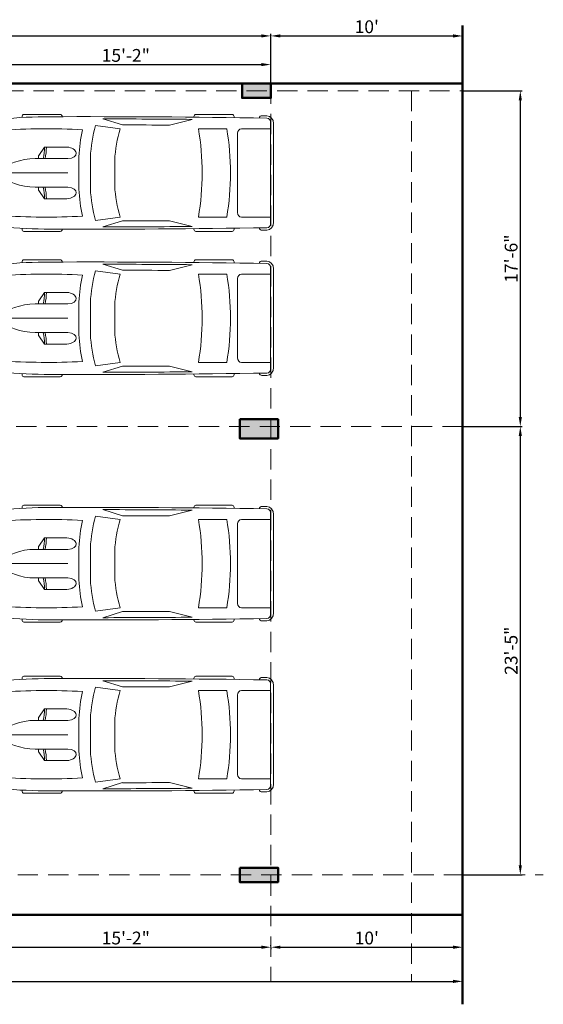
# Model space of a CAD drawing. Units: millimetres. Extents: x 1706 to 5913, y 156 to 1716.
# Tile 7 of 26: x 2350 to 2678, y 1086 to 1702. Entities that reach past the tile are written whole.
import ezdxf

# ---------------------------------------------------------------- set-up
doc = ezdxf.new("R2010")
doc.units = ezdxf.units.MM
doc.linetypes.add('DASHED', pattern=[19.05, 12.7, -6.35])
for name, color, linetype, lineweight in [('A-ANNO-DIMS', 2, 'Continuous', 18), ('A-COLS', 20, 'Continuous', 50), ('A-EQPM', 8, 'Continuous', 18), ('A-FLOR-OVHD', 9, 'DASHED', 18), ('A-WALL', 7, 'Continuous', 50)]:
    doc.layers.add(name, color=color, linetype=linetype, lineweight=lineweight)
doc.styles.get("Standard").update_dxf_attribs({"font": 'arial.ttf'})
doc.dimstyles.new('ISO-25', dxfattribs={"dimtxt": 8, "dimasz": 6, "dimexe": 1.25, "dimexo": 0.625, "dimtad": 1, "dimdec": 0, "dimlunit": 3, "dimtxsty": 'Standard', "dimcen": 2.5, "dimadec": 0, "dimazin": 0, "dimtfac": 1, "dimtdec": 0, "dimtmove": 0, "dimatfit": 3, "dimfxl": 1, "dimarcsym": 0})

# ---------------------------------------------------------------- blocks, each defined once
blk = doc.blocks.new('*U10')
for p, q in [((21.1, 37.41), (21.1, 36.83)), ((46.55, 38.89), (22.35, 38.89)), ((47.8, 37.39), (47.8, 37.41)), ((87.99, 31.87), (74.76, 35.92)), ((134.31, 35.6), (119.29, 31.78)), ((135.45, 37.07), (135.45, 37.41)), ((136.7, 38.89), (160.9, 38.89)), ((162.15, 37.41), (162.15, 36.77)), ((186.47, -33.5), (186.47, 33.5)), ((188.4, -32.76), (188.4, 32.76)), ((70.03, 31.54), (86.41, 29.35)), ((138.42, 29.35), (157.25, 29.35)), ((164.52, 26.39), (164.52, -26.39)), ((186.47, 29.35), (167.01, 29.35)), ((32.27, 11.63), (36.13, 17.17)), ((36.13, 17.17), (50.94, 17.17)), ((29.77, 9.51), (51.68, 9.51)), ((32.12, 9.51), (32.12, 11.15)), ((58.92, -10.77), (58.92, 10.77)), ((66.55, -10.53), (66.55, 10.53)), ((82.74, 8.5), (82.74, -8.5)), ((186.47, -10.53), (186.47, 10.53)), ((3.27, 6.13), (0.1, 0.41)), ((0, 0), (51.68, 0)), ((0.1, -0.41), (3.27, -6.13)), ((29.77, -9.51), (51.68, -9.51)), ((32.12, -9.51), (32.12, -11.15)), ((32.27, -11.63), (36.13, -17.17)), ((36.13, -17.17), (50.94, -17.17)), ((86.41, -29.35), (70.03, -31.54)), ((87.99, -31.87), (74.76, -35.92)), ((134.31, -35.6), (119.29, -31.78)), ((157.25, -29.35), (138.42, -29.35)), ((167.01, -29.35), (186.47, -29.35)), ((21.1, -37.41), (21.1, -36.83)), ((46.55, -38.89), (22.35, -38.89)), ((47.8, -37.39), (47.8, -37.41)), ((135.45, -37.07), (135.45, -37.41)), ((136.7, -38.89), (160.9, -38.89)), ((162.15, -37.41), (162.15, -36.77))]:
    blk.add_line(p, q)
for centre, major_axis, ratio, start_param, end_param in [((266.03, -27.52), (0, 313.31), 0.842304, 1.367076, 1.39176), ((41.19, -490.86), (0, 528.23), 0.842304, 0.00281, 0.075598), ((22.35, 37.41), (0, -1.48), 0.842304, 3.141593, 4.712389), ((64.48, -10555.62), (0, 10593.03), 0.842304, -0.013397, 0.002797), ((46.55, 37.41), (0, 1.48), 0.842304, -1.570796, 0), ((64.48, -10555.62), (0, -10591.55), 0.842304, 3.133765, 3.140441), ((136.7, 37.41), (0, -1.48), 0.842304, 3.141593, 4.712389), ((160.9, 37.41), (0, 1.48), 0.842304, -1.570796, 0), ((180.63, 35.84), (0, 2.22), 0.842304, -0.013017, 1.249894), ((64.48, -10556.36), (0, 10595.31), 0.842304, -0.013397, -0.013017), ((183.98, 33.5), (0, -2.96), 0.842304, 1.570796, 3.128196), ((183.98, 32.76), (0, -5.25), 0.842304, 1.570796, 3.128196), ((259.18, -27.52), (0, -305.3), 0.842304, 4.528606, 4.561838), ((37.47, -593.96), (0, -623.33), 0.842304, 3.096046, 3.200911), ((134.4, 5.39), (0, -89.78), 0.842304, 4.449482, 4.652344), ((135.29, 5.39), (0, 81.77), 0.842304, 1.245306, 1.50788), ((149.6, 2.8), (0, -79.58), 0.842304, 4.372215, 4.640744), ((95.79, -3666.35), (0, -3698.24), 0.842304, 3.134049, 3.144098), ((17.08, 0), (0, 147.02), 0.842304, 4.511394, 4.913384), ((35.91, 0), (0, 147.02), 0.842304, 4.511394, 4.913384), ((167.01, 26.39), (0, 2.96), 0.842304, 0, 1.570796), ((-204.49, 52.4), (0, -250.96), 0.842304, 1.385369, 1.434372), ((13.04, 17.01), (0, 27.42), 0.842304, 4.435146, 4.718221), ((14.2, 17.01), (0, 27.42), 0.842304, 4.435146, 4.718221), ((50.79, 13.34), (6.34, -0.36), 0.603834, -1.395552, 1.581315), ((29.77, -46.66), (0, 56.17), 0.842304, 0, 0.590319), ((32.75, 11.15), (0, 0.74), 0.842304, 0.879714, 1.570796), ((0.62, 0), (0, -0.74), 0.842304, 4.131459, 5.293319), ((-204.49, -52.4), (0, 250.96), 0.842304, -1.434372, -1.385369), ((29.77, 46.66), (0, 56.17), 0.842304, 2.551274, 3.141593), ((32.75, -11.15), (0, -0.74), 0.842304, 4.712389, 5.403472), ((13.04, -17.01), (0, -27.42), 0.842304, 1.564964, 1.848039), ((14.2, -17.01), (0, -27.42), 0.842304, 1.564964, 1.848039), ((134.4, -5.39), (0, -89.78), 0.842304, -1.510751, -1.307889), ((135.29, -5.39), (0, -81.77), 0.842304, -1.50788, -1.245306), ((149.6, -2.8), (0, -79.58), 0.842304, -1.499151, -1.230623), ((259.18, 27.52), (0, 305.3), 0.842304, 1.721348, 1.754579), ((266.03, 27.52), (0, 313.31), 0.842304, 1.749832, 1.774517), ((37.47, 593.96), (0, -623.33), 0.842304, -0.059319, 0.045547), ((95.79, 3666.35), (0, -3698.24), 0.842304, -0.002505, 0.007544), ((167.01, -26.39), (0, -2.96), 0.842304, 4.712389, 6.283185), ((41.19, 490.86), (0, -528.23), 0.842304, -0.075598, -0.00281), ((22.35, -37.41), (0, 1.48), 0.842304, 1.570796, 3.141593), ((64.48, 10555.62), (0, 10593.03), 0.842304, 3.138796, 3.15499), ((46.55, -37.41), (0, -1.48), 0.842304, 0, 1.570796), ((64.48, 10555.62), (0, -10591.55), 0.842304, 0.001152, 0.007828), ((136.7, -37.41), (0, -1.48), 0.842304, -1.570796, 0), ((160.9, -37.41), (0, 1.48), 0.842304, 3.141593, 4.712389), ((180.63, -35.84), (0, -2.22), 0.842304, -1.249894, 0.013017), ((64.48, 10556.36), (0, 10595.31), 0.842304, 3.15461, 3.15499), ((183.98, -33.5), (0, 2.96), 0.842304, 3.15499, 4.712389), ((183.98, -32.76), (0, -5.25), 0.842304, 0.013397, 1.570796)]:
    blk.add_ellipse(centre, major_axis=major_axis, ratio=ratio, start_param=start_param, end_param=end_param)
at = {"extrusion": (0, 0, -1)}
blk.add_ellipse((50.79, -13.34), major_axis=(6.34, 0.36), ratio=0.603834, start_param=-1.395552, end_param=1.581315, dxfattribs=at)
blk = doc.blocks.new('*D90')
at = {"layer": 'A-ANNO-DIMS', "color": 0, "lineweight": -2, "transparency": 16777216}
for p, q in [((2325.9, 1122.72), (2325.9, 1123.34)), ((2331.9, 1122.09), (2501.4, 1122.09)), ((2507.4, 1122.72), (2507.4, 1123.34))]:
    blk.add_line(p, q, dxfattribs=at)
at = {"layer": 'A-ANNO-DIMS', "color": 0, "transparency": 16777216}
for points in [[(2331.9, 1123.09), (2331.9, 1121.09), (2325.9, 1122.09)], [(2501.4, 1123.09), (2501.4, 1121.09), (2507.4, 1122.09)]]:
    blk.add_solid(points, dxfattribs=at)
at = {"layer": 'Defpoints', "color": 0, "transparency": 16777216}
for p in [(2325.9, 1122.09), (2507.4, 1122.09), (2507.4, 1122.09)]:
    blk.add_point(p, dxfattribs=at)
at = {"layer": 'A-ANNO-DIMS', "color": 0, "transparency": 16777216, "insert": (2416.65, 1126.8), "char_height": 8, "attachment_point": 5}
blk.add_mtext('15\'-2"', dxfattribs=at)
blk = doc.blocks.new('*D91')
at = {"layer": 'A-ANNO-DIMS', "color": 0, "lineweight": -2, "transparency": 16777216}
for p, q in [((2507.4, 1121.47), (2507.4, 1120.84)), ((2513.4, 1122.09), (2621.4, 1122.09)), ((2627.4, 1123.72), (2627.4, 1120.84))]:
    blk.add_line(p, q, dxfattribs=at)
at = {"layer": 'A-ANNO-DIMS', "color": 0, "transparency": 16777216}
for points in [[(2513.4, 1123.09), (2513.4, 1121.09), (2507.4, 1122.09)], [(2621.4, 1123.09), (2621.4, 1121.09), (2627.4, 1122.09)]]:
    blk.add_solid(points, dxfattribs=at)
at = {"layer": 'Defpoints', "color": 0, "transparency": 16777216}
for p in [(2507.4, 1122.09), (2627.4, 1124.34), (2627.4, 1122.09)]:
    blk.add_point(p, dxfattribs=at)
at = {"layer": 'A-ANNO-DIMS', "color": 0, "transparency": 16777216, "insert": (2567.4, 1126.8), "char_height": 8, "attachment_point": 5}
blk.add_mtext("10'", dxfattribs=at)
blk = doc.blocks.new('*D96')
at = {"layer": 'A-ANNO-DIMS', "color": 0, "lineweight": -2, "transparency": 16777216}
for p, q in [((2325.9, 1662.9), (2325.9, 1675.38)), ((2507.4, 1662.9), (2507.4, 1675.38)), ((2331.9, 1674.13), (2501.4, 1674.13))]:
    blk.add_line(p, q, dxfattribs=at)
at = {"layer": 'A-ANNO-DIMS', "color": 0, "transparency": 16777216}
for points in [[(2331.9, 1675.13), (2331.9, 1673.13), (2325.9, 1674.13)], [(2501.4, 1675.13), (2501.4, 1673.13), (2507.4, 1674.13)]]:
    blk.add_solid(points, dxfattribs=at)
at = {"layer": 'Defpoints', "color": 0, "transparency": 16777216}
for p in [(2507.4, 1674.13), (2325.9, 1662.28), (2507.4, 1662.28)]:
    blk.add_point(p, dxfattribs=at)
at = {"layer": 'A-ANNO-DIMS', "color": 0, "transparency": 16777216, "insert": (2416.65, 1678.84), "char_height": 8, "attachment_point": 5}
blk.add_mtext('15\'-2"', dxfattribs=at)
blk = doc.blocks.new('*D83')
at = {"layer": 'A-ANNO-DIMS', "color": 0, "lineweight": -2, "transparency": 16777216}
for p, q in [((2507.4, 1692.67), (2507.4, 1693.3)), ((2513.4, 1692.05), (2621.4, 1692.05)), ((2627.4, 1692.67), (2627.4, 1693.3))]:
    blk.add_line(p, q, dxfattribs=at)
at = {"layer": 'A-ANNO-DIMS', "color": 0, "transparency": 16777216}
for points in [[(2513.4, 1693.05), (2513.4, 1691.05), (2507.4, 1692.05)], [(2621.4, 1693.05), (2621.4, 1691.05), (2627.4, 1692.05)]]:
    blk.add_solid(points, dxfattribs=at)
at = {"layer": 'Defpoints', "color": 0, "transparency": 16777216}
for p in [(2507.4, 1692.05), (2627.4, 1692.05), (2627.4, 1692.05)]:
    blk.add_point(p, dxfattribs=at)
at = {"layer": 'A-ANNO-DIMS', "color": 0, "transparency": 16777216, "insert": (2567.4, 1696.76), "char_height": 8, "attachment_point": 5}
blk.add_mtext("10'", dxfattribs=at)
blk = doc.blocks.new('*D99')
at = {"layer": 'A-ANNO-DIMS', "color": 0, "lineweight": -2, "transparency": 16777216}
for p, q in [((1739.4, 1141.65), (1739.4, 1099.48)), ((2627.4, 1141.65), (2627.4, 1099.48)), ((1745.4, 1100.73), (2621.4, 1100.73))]:
    blk.add_line(p, q, dxfattribs=at)
at = {"layer": 'A-ANNO-DIMS', "color": 0, "transparency": 16777216}
for points in [[(1745.4, 1101.73), (1745.4, 1099.73), (1739.4, 1100.73)], [(2621.4, 1101.73), (2621.4, 1099.73), (2627.4, 1100.73)]]:
    blk.add_solid(points, dxfattribs=at)
at = {"layer": 'Defpoints', "color": 0, "transparency": 16777216}
for p in [(1739.4, 1142.28), (2627.4, 1142.28), (2627.4, 1100.73)]:
    blk.add_point(p, dxfattribs=at)
at = {"layer": 'A-ANNO-DIMS', "color": 0, "transparency": 16777216, "insert": (2183.4, 1105.35), "char_height": 8, "attachment_point": 5}
blk.add_mtext("74'", dxfattribs=at)
blk = doc.blocks.new('*D100')
at = {"layer": 'A-ANNO-DIMS', "color": 0, "lineweight": -2, "transparency": 16777216}
for p, q in [((1787.4, 1662.9), (1787.4, 1693.3)), ((1793.4, 1692.05), (2501.4, 1692.05)), ((2507.4, 1662.9), (2507.4, 1693.3))]:
    blk.add_line(p, q, dxfattribs=at)
at = {"layer": 'A-ANNO-DIMS', "color": 0, "transparency": 16777216}
for points in [[(1793.4, 1693.05), (1793.4, 1691.05), (1787.4, 1692.05)], [(2501.4, 1693.05), (2501.4, 1691.05), (2507.4, 1692.05)]]:
    blk.add_solid(points, dxfattribs=at)
at = {"layer": 'Defpoints', "color": 0, "transparency": 16777216}
for p in [(2507.4, 1692.05), (1787.4, 1662.28), (2507.4, 1662.28)]:
    blk.add_point(p, dxfattribs=at)
at = {"layer": 'A-ANNO-DIMS', "color": 0, "transparency": 16777216, "insert": (2147.4, 1696.76), "char_height": 8, "attachment_point": 5}
blk.add_mtext("60'", dxfattribs=at)
blk = doc.blocks.new('*D104')
at = {"layer": 'A-ANNO-DIMS', "color": 0, "lineweight": -2, "transparency": 16777216}
for p, q in [((2628.03, 1657.78), (2664.72, 1657.78)), ((2663.47, 1651.78), (2663.47, 1453.78)), ((2628.03, 1447.78), (2664.72, 1447.78))]:
    blk.add_line(p, q, dxfattribs=at)
at = {"layer": 'A-ANNO-DIMS', "color": 0, "transparency": 16777216}
for points in [[(2662.47, 1651.78), (2664.47, 1651.78), (2663.47, 1657.78)], [(2662.47, 1453.78), (2664.47, 1453.78), (2663.47, 1447.78)]]:
    blk.add_solid(points, dxfattribs=at)
at = {"layer": 'Defpoints', "color": 0, "transparency": 16777216}
for p in [(2627.4, 1657.78), (2627.4, 1447.78), (2663.47, 1447.78)]:
    blk.add_point(p, dxfattribs=at)
at = {"layer": 'A-ANNO-DIMS', "color": 0, "transparency": 16777216, "insert": (2658.76, 1552.78), "char_height": 8, "attachment_point": 5, "rotation": 90}
blk.add_mtext('17\'-6"', dxfattribs=at)
blk = doc.blocks.new('*D105')
at = {"layer": 'A-ANNO-DIMS', "color": 0, "lineweight": -2, "transparency": 16777216}
for p, q in [((2628.03, 1447.78), (2664.72, 1447.78)), ((2663.47, 1441.78), (2663.47, 1173.28)), ((2628.03, 1167.28), (2664.72, 1167.28))]:
    blk.add_line(p, q, dxfattribs=at)
at = {"layer": 'A-ANNO-DIMS', "color": 0, "transparency": 16777216}
for points in [[(2662.47, 1441.78), (2664.47, 1441.78), (2663.47, 1447.78)], [(2662.47, 1173.28), (2664.47, 1173.28), (2663.47, 1167.28)]]:
    blk.add_solid(points, dxfattribs=at)
at = {"layer": 'Defpoints', "color": 0, "transparency": 16777216}
for p in [(2627.4, 1447.78), (2627.4, 1167.28), (2663.47, 1167.28)]:
    blk.add_point(p, dxfattribs=at)
at = {"layer": 'A-ANNO-DIMS', "color": 0, "transparency": 16777216, "insert": (2658.76, 1307.53), "char_height": 8, "attachment_point": 5, "rotation": 90}
blk.add_mtext('23\'-5"', dxfattribs=at)

msp = doc.modelspace()

# ---------------------------------------------------------------- hatches: boundary and pattern name
at = {"layer": 'A-COLS'}
h = msp.add_hatch(color=256, dxfattribs=at)
h.dxf.hatch_style = 1
h.paths.add_polyline_path([(2507.4, 1662.28), (2489.4, 1662.28), (2489.4, 1653.28), (2507.4, 1653.28)])
h = msp.add_hatch(color=256, dxfattribs=at)
h.dxf.hatch_style = 1
h.paths.add_polyline_path([(2511.9, 1452.28), (2487.9, 1452.28), (2487.9, 1440.28), (2511.9, 1440.28)])
h = msp.add_hatch(color=256, dxfattribs=at)
h.dxf.hatch_style = 1
h.paths.add_polyline_path([(2511.9, 1171.78), (2487.9, 1171.78), (2487.9, 1162.78), (2511.9, 1162.78)])

# ---------------------------------------------------------------- linework, layer by layer
for points in [[(2507.4, 1662.28), (2489.4, 1662.28), (2489.4, 1653.28), (2507.4, 1653.28)], [(2487.9, 1452.28), (2511.9, 1452.28), (2511.9, 1440.28), (2487.9, 1440.28)], [(2487.9, 1171.78), (2511.9, 1171.78), (2511.9, 1162.78), (2487.9, 1162.78)]]:
    msp.add_lwpolyline(points, close=True, dxfattribs=at)
at = {"layer": 'A-FLOR-OVHD'}
for p, q in [((1787.4, 1657.78), (2627.4, 1657.78)), ((2507.4, 1662.28), (2507.4, 1101.1)), ((2595.31, 1657.78), (2595.31, 1101.1)), ((2627.4, 1447.78), (2174.4, 1447.78)), ((1739.4, 1167.28), (2677.86, 1167.28))]:
    msp.add_line(p, q, dxfattribs=at)
at = {"layer": 'A-WALL'}
for p, q in [((2627.4, 1086.38), (2627.4, 1698.62)), ((2343.9, 1662.28), (2627.4, 1662.28)), ((2627.4, 1142.28), (1739.4, 1142.28))]:
    msp.add_line(p, q, dxfattribs=at)

# ---------------------------------------------------------------- block references
at = {"layer": 'A-EQPM', "xscale": 0.9406440953584901, "yscale": 0.9406440953584901, "zscale": 0.9406440953584901}
for p in [(2331.86, 1606.37), (2331.86, 1515.48), (2331.86, 1361.99), (2331.86, 1254.99)]:
    msp.add_blockref('*U10', p, dxfattribs=at)

# ---------------------------------------------------------------- dimensions: what is measured, and where the dimension line sits
at = {"layer": 'A-ANNO-DIMS'}
for base, p1, p2, picture, middle in [((2507.4, 1692.05), (1787.4, 1662.28), (2507.4, 1662.28), '*D100', (2147.4, 1696.76)), ((2627.4, 1692.05), (2507.4, 1692.05), (2627.4, 1692.05), '*D83', (2567.4, 1696.76)), ((2507.4015753, 1674.12925326), (2325.9015753, 1662.27547118), (2507.4015753, 1662.27547118), '*D96', (2416.6515753, 1678.83883716)), ((2627.4, 1100.73), (1739.4, 1142.28), (2627.4, 1142.28), '*D99', (2183.4, 1105.35)), ((2507.4015753, 1122.09031597), (2325.9015753, 1122.09031597), (2507.4015753, 1122.09031597), '*D90', (2416.6515753, 1126.79989987)), ((2627.4, 1122.09), (2507.4, 1122.09), (2627.4, 1124.34), '*D91', (2567.4, 1126.8))]:
    dim = msp.add_linear_dim(base=base, p1=p1, p2=p2, dimstyle='ISO-25', override={"dimclrd": 0, "dimclre": 0, "dimclrt": 0}, dxfattribs=at)
    dim.commit()
    dim.dimension.update_dxf_attribs({"geometry": picture, "text_midpoint": middle})
for base, p1, p2, picture, middle in [((2663.47, 1447.78), (2627.4, 1657.78), (2627.4, 1447.78), '*D104', (2658.76, 1552.78)), ((2663.46988962, 1167.27547118), (2627.4015753, 1447.77547118), (2627.4015753, 1167.27547118), '*D105', (2658.7575772, 1307.52547118))]:
    dim = msp.add_linear_dim(base=base, p1=p1, p2=p2, angle=90, dimstyle='ISO-25', override={"dimclrd": 0, "dimclre": 0, "dimclrt": 0}, dxfattribs=at)
    dim.commit()
    dim.dimension.update_dxf_attribs({"geometry": picture, "text_midpoint": middle})

doc.saveas('drawing.dxf')
